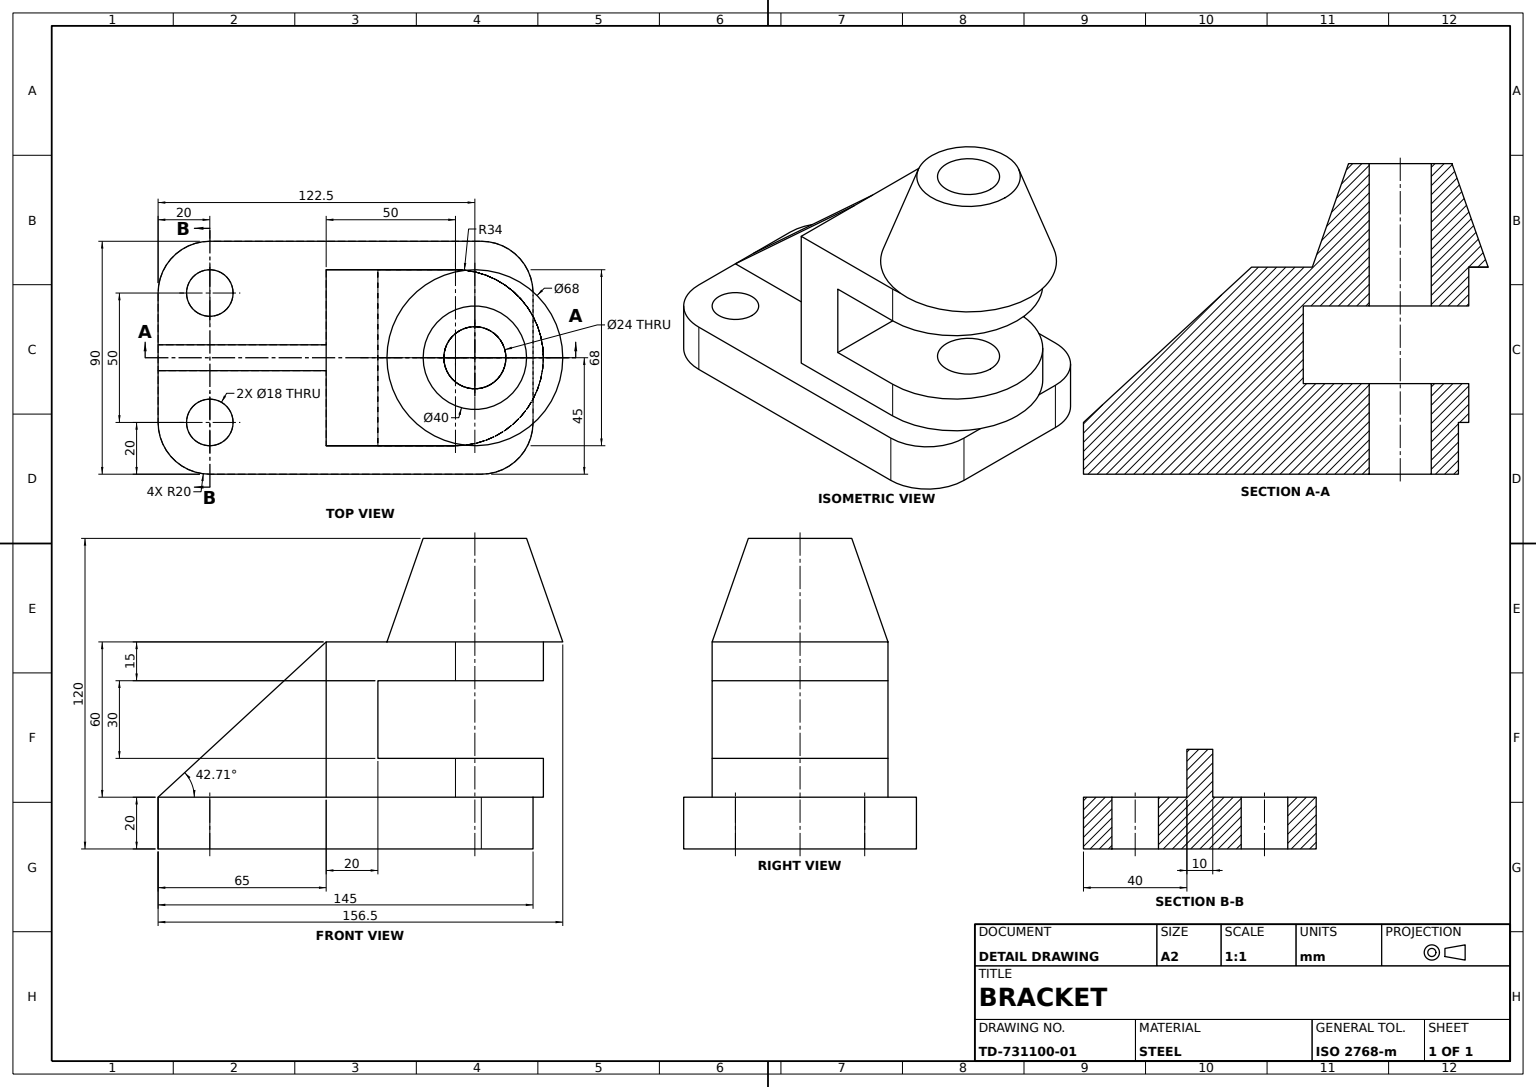
from build123d import *

# Parameters (mm, degrees)
BASE_PLATE_SKETCH_W       = 90
BASE_PLATE_SKETCH_H       = 145
BASE_PLATE_SKETCH_R       = 9
BASE_PLATE_DEPTH          = 20
BASE_CORNER_FILLETS_R20_R = 20
UPRIGHT_BLOCK_DEPTH       = 60
SIDE_START                = -45
SIDE_SLOT_DEPTH           = 30
CONE_BORE_SKETCH_R        = 12
CONE_BORE_24_DEPTH        = 154.235113469
SUPPORT_RIB_10MM_REACH    = 155.235
SUPPORT_RIB_SKETCH_WALL_W = 396.929257004
SUPPORT_RIB_SKETCH_WALL_H = 10


with BuildPart() as part:
    # Base Plate Sketch → Base Plate (new body)
    with BuildSketch(Plane(origin=(0, 0, 0), x_dir=(1, 0, 0), z_dir=(0, 1, 0))):
        Rectangle(BASE_PLATE_SKETCH_W, BASE_PLATE_SKETCH_H)
        with Locations(Location((-25, -52.5, 0), (0, 0, 270))):
            Circle(BASE_PLATE_SKETCH_R, mode=Mode.SUBTRACT)
        with Locations(Location((25, -52.5, 0), (0, 0, 270))):
            Circle(BASE_PLATE_SKETCH_R, mode=Mode.SUBTRACT)
    extrude(amount=BASE_PLATE_DEPTH)

    # Base Corner Fillets R20
    base_corner_fillets_r20_edges = [part.edges().sort_by_distance(p)[0] for p in [
        (-45, 10, -72.5),
        (45, 10, -72.5),
        (45, 10, 72.5),
        (-45, 10, 72.5),
    ]]
    fillet(base_corner_fillets_r20_edges, radius=BASE_CORNER_FILLETS_R20_R)

    # Upright Block Sketch → Upright Block (add)
    with BuildSketch(Plane(origin=(0, 20, 0), x_dir=(1, 0, 0), z_dir=(0, 1, 0))):
        with BuildLine():
            Line((-34, -7.5), (34, -7.5))
            Line((34, -7.5), (34, 42.5))
            ThreePointArc((34, 42.5), (0, 76.5), (-34, 42.5))
            Line((-34, 42.5), (-34, -7.5))
        make_face()
    extrude(amount=UPRIGHT_BLOCK_DEPTH)

    # Side Slot Sketch → Side Slot (cut)
    with BuildSketch(Plane(origin=(0, 80, 0), x_dir=(1, 0, 0), z_dir=(0, 1, 0)).offset(SIDE_START)):
        with BuildLine():
            Line((-34, 42.5), (-34, 12.5))
            Line((-34, 12.5), (34, 12.5))
            Line((34, 12.5), (34, 42.5))
            ThreePointArc((34, 42.5), (0, 76.5), (-34, 42.5))
        make_face()
    extrude(amount=SIDE_SLOT_DEPTH, mode=Mode.SUBTRACT)

    # Cone Boss Profile → Cone Boss (revolve)
    with BuildSketch(Plane.XY.offset(-50), mode=Mode.PRIVATE) as cone_boss_sk:
        Polygon((0, 80), (0, 120), (20, 120), (34, 80), align=None)
    revolve(cone_boss_sk.sketch.rotate(Axis((0, 80, -50), (0, 1, 0)), 90), axis=Axis((0, 80, -50), (0, 1, 0)))

    # Cone Bore Sketch → Cone Bore Ø24 (cut, through all)
    with BuildSketch(Plane(origin=(0, 120, 0), x_dir=(1, 0, 0), z_dir=(0, 1, 0))):
        with Locations(Location((0, 50, 0), (0, 0, 270))):
            Circle(CONE_BORE_SKETCH_R)
    extrude(amount=-CONE_BORE_24_DEPTH, mode=Mode.SUBTRACT)

    # Support Rib Sketch wall → Support Rib 10mm (add, up to next)
    with BuildSketch(Plane(origin=(0, 50, 40), x_dir=(0, 0.678280102733, -0.734803444627), z_dir=(0, 0.734803444627, 0.678280102733)), mode=Mode.PRIVATE) as support_rib_10mm_sk1:
        Rectangle(SUPPORT_RIB_SKETCH_WALL_W, SUPPORT_RIB_SKETCH_WALL_H)
    support_rib_10mm_tool1 = extrude(support_rib_10mm_sk1.sketch, amount=-SUPPORT_RIB_10MM_REACH, mode=Mode.PRIVATE) - part.part
    add(support_rib_10mm_tool1.solids().sort_by_distance((0, 50, 40))[0])


solid = part.part
